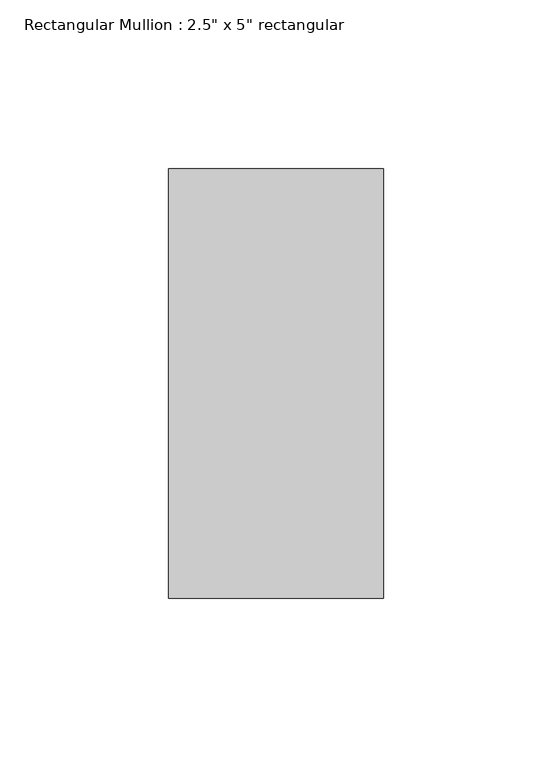
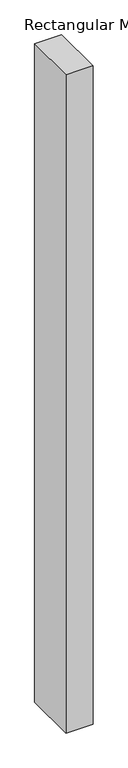
"""IFC4 building model written with IfcOpenShell, lengths in millimetres: member geometry."""

from ifc_helpers import new_model, si_unit, frame, origin, place, context, project, spatial, polyline, outline, extrude, source, transform, mapped, element, save


def member_0bc49b9d(model_context):
    return source(origin(), model_context, "Body", "SweptSolid", [
        extrude(outline(polyline([(31.75, 63.5), (31.75, -63.5), (-31.75, -63.5), (-31.75, 63.5), (31.75, 63.5)])), frame((0.0, 0.0, -1633.9367938), z_axis=(0.0, 0.0, 1.0), x_axis=(1.0, 0.0, 0.0)), (0.0, 0.0, 1.0), 1633.9367938),
    ])


if __name__ == "__main__":
    model = new_model("IFC4")
    model_context = context("Model", 3, world=origin())
    ifc_project = project(units=[si_unit("LENGTHUNIT", "METRE", prefix="MILLI")], contexts=[model_context])
    site = spatial("IfcSite", under=ifc_project)
    building = spatial("IfcBuilding", under=site)
    placement = place(None, origin())
    member_shape = member_0bc49b9d(model_context)
    element("IfcMember", 1, ObjectType="Rectangular Mullion : 2.5\" x 5\" rectangular", at=placement, inside=building, context=model_context, shape_type="MappedRepresentation", body=[
        mapped(member_shape, transform((0.0, 0.0, 0.0), x_axis=(1.0, 0.0, 0.0), y_axis=(0.0, 1.0, 0.0), z_axis=(0.0, 0.0, 1.0))),
    ])
    save(model, "model.ifc")

# Revit data of these elements
# Type "Rectangular Mullion : 2.5\" x 5\" rectangular"
#   built-in parameter 1007304 = 0.416667 (stored number, unit not read)
#   built-in parameter 1007301 = 0.104167 (stored number, unit not read)
#   built-in parameter 1007300 = 0.104167 (stored number, unit not read)
# Element 1 (IfcMember, "Rectangular Mullion : 2.5\" x 5\" rectangular")
#   Materials on its faces: "Aluminum"
# Materials
#   "Aluminum": class "Metal", colour RGB 247 247 247, transparency 0, Description = "Aluminum 6061", Cost = 0
